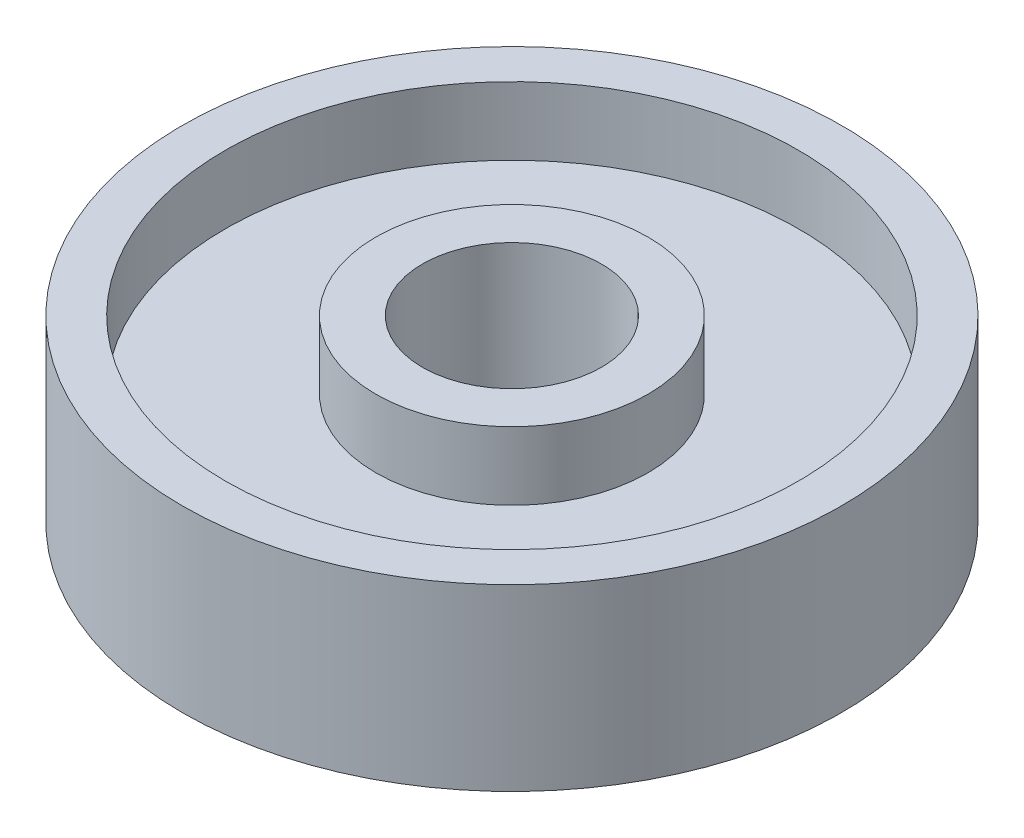
from build123d import *

# Parameters (mm, degrees)
BASE_DISC_SKETCH_R = 46
BASE_DISC_92_DEPTH = 3
RIM_START          = 9.5
RIM_SKETCH_R       = 46
RIM_SKETCH_R_2     = 40
RIM_92X_80_DEPTH   = 9.5
HUB_SKETCH_R       = 19
HUB_SKETCH_R_2     = 12.5
HUB_38_DEPTH       = 25
BORE_SKETCH_R      = 12.5
BORE_25_DEPTH      = 25


with BuildPart() as part:
    # Base Disc Sketch → Base Disc Ø92 (new, symmetric)
    with BuildSketch(Plane(origin=(0, 0, 0), x_dir=(1, 0, 0), z_dir=(0, 1, 0))):
        with Locations(Location((0, 0, 0), (0, 0, 270))):
            Circle(BASE_DISC_SKETCH_R)
    extrude(amount=BASE_DISC_92_DEPTH, both=True)

    # Rim Sketch → Rim Ø92xØ80 (add)
    with BuildSketch(Plane(origin=(0, 3, 0), x_dir=(1, 0, 0), z_dir=(0, 1, 0)).offset(RIM_START)):
        with Locations(Location((0, 0, 0), (0, 0, 270))):
            Circle(RIM_SKETCH_R)
        with Locations(Location((0, 0, 0), (0, 0, 270))):
            Circle(RIM_SKETCH_R_2, mode=Mode.SUBTRACT)
    rim_92x_80 = extrude(amount=-RIM_92X_80_DEPTH)

    # Rim Mirror: Rim Ø92xØ80 across plane
    add(rim_92x_80.mirror(Plane.ZX))

    # Hub Sketch → Hub Ø38 (add)
    with BuildSketch(Plane(origin=(0, 12.5, 0), x_dir=(1, 0, 0), z_dir=(0, 1, 0))):
        with Locations(Location((0, 0, 0), (0, 0, 270))):
            Circle(HUB_SKETCH_R)
        with Locations(Location((0, 0, 0), (0, 0, 270))):
            Circle(HUB_SKETCH_R_2, mode=Mode.SUBTRACT)
    extrude(amount=-HUB_38_DEPTH)

    # Bore Sketch → Bore Ø25 (cut)
    with BuildSketch(Plane(origin=(0, 3, 0), x_dir=(1, 0, 0), z_dir=(0, 1, 0))):
        with Locations(Location((0, 0, 0), (0, 0, 270))):
            Circle(BORE_SKETCH_R)
    extrude(amount=-BORE_25_DEPTH, mode=Mode.SUBTRACT)


solid = part.part
